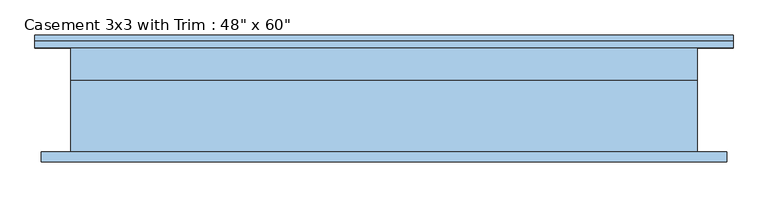
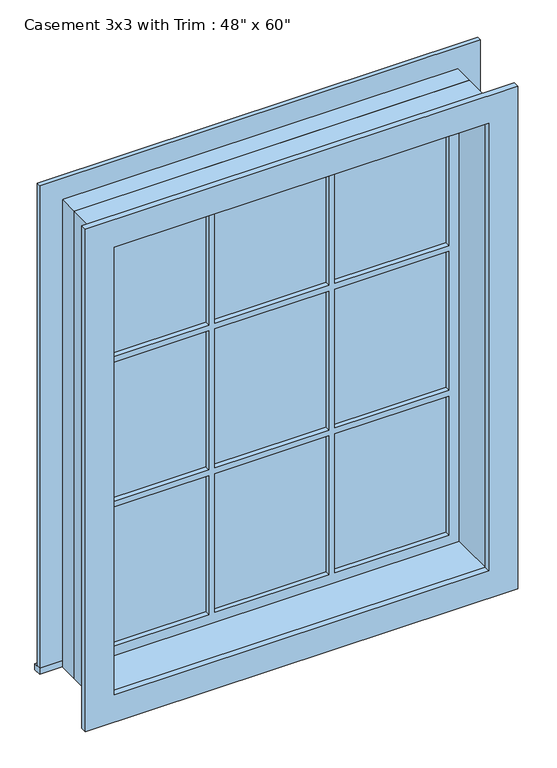
"""IFC4 building model written with IfcOpenShell, lengths in millimetres: window geometry."""

from ifc_helpers import new_model, si_unit, frame, origin, place, context, project, spatial, polyline, outline, extrude, source, transform, mapped, element, save


def window_cfa1ffdd(model_context):
    return source(origin(), model_context, "Body", "SweptSolid", [
        extrude(outline(polyline([(-679.45, 127.0), (679.45, 127.0), (679.45, 101.6), (-679.45, 101.6), (-679.45, 127.0)])), frame((0.0, 0.0, 609.6), z_axis=(0.0, 0.0, 1.0), x_axis=(1.0, 0.0, 0.0)), (0.0, 0.0, 1.0), 19.05),
        extrude(outline(polyline([(2114.55, -590.55), (2114.55, 590.55), (628.65, 590.55), (628.65, 679.45), (2203.45, 679.45), (2203.45, -679.45), (628.65, -679.45), (628.65, -590.55), (2114.55, -590.55)])), frame((0.0, 101.6, 0.0), z_axis=(0.0, 1.0, 0.0), x_axis=(0.0, 0.0, 1.0)), (0.0, 0.0, 1.0), 12.7),
        extrude(outline(polyline([(194.7333333, 66.675), (546.1, 66.675), (546.1, 53.975), (194.7333333, 53.975), (194.7333333, 66.675)])), frame((0.0, 0.0, 1617.1333333), z_axis=(0.0, 0.0, 1.0), x_axis=(1.0, 0.0, 0.0)), (0.0, 0.0, 1.0), 452.9666667),
        extrude(outline(polyline([(-175.6833333, 66.675), (175.6833333, 66.675), (175.6833333, 53.975), (-175.6833333, 53.975), (-175.6833333, 66.675)])), frame((0.0, 0.0, 1617.1333333), z_axis=(0.0, 0.0, 1.0), x_axis=(1.0, 0.0, 0.0)), (0.0, 0.0, 1.0), 452.9666667),
        extrude(outline(polyline([(-546.1, 66.675), (-194.7333333, 66.675), (-194.7333333, 53.975), (-546.1, 53.975), (-546.1, 66.675)])), frame((0.0, 0.0, 1617.1333333), z_axis=(0.0, 0.0, 1.0), x_axis=(1.0, 0.0, 0.0)), (0.0, 0.0, 1.0), 452.9666667),
        extrude(outline(polyline([(-546.1, 66.675), (-194.7333333, 66.675), (-194.7333333, 53.975), (-546.1, 53.975), (-546.1, 66.675)])), frame((0.0, 0.0, 1145.1166667), z_axis=(0.0, 0.0, 1.0), x_axis=(1.0, 0.0, 0.0)), (0.0, 0.0, 1.0), 452.9666667),
        extrude(outline(polyline([(-175.6833333, 66.675), (175.6833333, 66.675), (175.6833333, 53.975), (-175.6833333, 53.975), (-175.6833333, 66.675)])), frame((0.0, 0.0, 1145.1166667), z_axis=(0.0, 0.0, 1.0), x_axis=(1.0, 0.0, 0.0)), (0.0, 0.0, 1.0), 452.9666667),
        extrude(outline(polyline([(194.7333333, 66.675), (546.1, 66.675), (546.1, 53.975), (194.7333333, 53.975), (194.7333333, 66.675)])), frame((0.0, 0.0, 1145.1166667), z_axis=(0.0, 0.0, 1.0), x_axis=(1.0, 0.0, 0.0)), (0.0, 0.0, 1.0), 452.9666667),
        extrude(outline(polyline([(194.7333333, 66.675), (546.1, 66.675), (546.1, 53.975), (194.7333333, 53.975), (194.7333333, 66.675)])), frame((0.0, 0.0, 673.1), z_axis=(0.0, 0.0, 1.0), x_axis=(1.0, 0.0, 0.0)), (0.0, 0.0, 1.0), 452.9666667),
        extrude(outline(polyline([(-175.6833333, 66.675), (175.6833333, 66.675), (175.6833333, 53.975), (-175.6833333, 53.975), (-175.6833333, 66.675)])), frame((0.0, 0.0, 673.1), z_axis=(0.0, 0.0, 1.0), x_axis=(1.0, 0.0, 0.0)), (0.0, 0.0, 1.0), 452.9666667),
        extrude(outline(polyline([(-546.1, 66.675), (-194.7333333, 66.675), (-194.7333333, 53.975), (-546.1, 53.975), (-546.1, 66.675)])), frame((0.0, 0.0, 673.1), z_axis=(0.0, 0.0, 1.0), x_axis=(1.0, 0.0, 0.0)), (0.0, 0.0, 1.0), 452.9666667),
        extrude(outline(polyline([(2190.75, 666.75), (2190.75, -666.75), (552.45, -666.75), (552.45, 666.75), (2190.75, 666.75)]), holes=[polyline([(2101.85, 577.85), (641.35, 577.85), (641.35, -577.85), (2101.85, -577.85), (2101.85, 577.85)])]), frame((0.0, -120.65, 0.0), z_axis=(0.0, 1.0, 0.0), x_axis=(0.0, 0.0, 1.0)), (0.0, 0.0, 1.0), 19.05),
        extrude(outline(polyline([(2114.55, -590.55), (628.65, -590.55), (628.65, 590.55), (2114.55, 590.55), (2114.55, -590.55)]), holes=[polyline([(2070.1, -194.7333333), (1617.1333333, -194.7333333), (1617.1333333, -546.1), (2070.1, -546.1), (2070.1, -194.7333333)]), polyline([(1598.0833333, -194.7333333), (1145.1166667, -194.7333333), (1145.1166667, -546.1), (1598.0833333, -546.1), (1598.0833333, -194.7333333)]), polyline([(1126.0666667, -194.7333333), (673.1, -194.7333333), (673.1, -546.1), (1126.0666667, -546.1), (1126.0666667, -194.7333333)]), polyline([(2070.1, 175.6833333), (1617.1333333, 175.6833333), (1617.1333333, -175.6833333), (2070.1, -175.6833333), (2070.1, 175.6833333)]), polyline([(1598.0833333, 175.6833333), (1145.1166667, 175.6833333), (1145.1166667, -175.6833333), (1598.0833333, -175.6833333), (1598.0833333, 175.6833333)]), polyline([(1126.0666667, 175.6833333), (673.1, 175.6833333), (673.1, -175.6833333), (1126.0666667, -175.6833333), (1126.0666667, 175.6833333)]), polyline([(2070.1, 546.1), (1617.1333333, 546.1), (1617.1333333, 194.7333333), (2070.1, 194.7333333), (2070.1, 546.1)]), polyline([(1598.0833333, 546.1), (1145.1166667, 546.1), (1145.1166667, 194.7333333), (1598.0833333, 194.7333333), (1598.0833333, 546.1)]), polyline([(1126.0666667, 546.1), (673.1, 546.1), (673.1, 194.7333333), (1126.0666667, 194.7333333), (1126.0666667, 546.1)])]), frame((0.0, 38.1, 0.0), z_axis=(0.0, 1.0, 0.0), x_axis=(0.0, 0.0, 1.0)), (0.0, 0.0, 1.0), 44.45),
        extrude(outline(polyline([(2133.6, -609.6), (609.6, -609.6), (609.6, 609.6), (2133.6, 609.6), (2133.6, -609.6)]), holes=[polyline([(2101.85, -577.85), (2101.85, 577.85), (641.35, 577.85), (641.35, -577.85), (2101.85, -577.85)])]), frame((0.0, -101.6, 0.0), z_axis=(0.0, 1.0, 0.0), x_axis=(0.0, 0.0, 1.0)), (0.0, 0.0, 1.0), 139.7),
        extrude(outline(polyline([(2133.6, 609.6), (2133.6, -609.6), (609.6, -609.6), (609.6, 609.6), (2133.6, 609.6)]), holes=[polyline([(2114.55, 590.55), (628.65, 590.55), (628.65, -590.55), (2114.55, -590.55), (2114.55, 590.55)])]), frame((0.0, 38.1, 0.0), z_axis=(0.0, 1.0, 0.0), x_axis=(0.0, 0.0, 1.0)), (0.0, 0.0, 1.0), 63.5),
    ])


if __name__ == "__main__":
    model = new_model("IFC4")
    model_context = context("Model", 3, world=origin())
    ifc_project = project(units=[si_unit("LENGTHUNIT", "METRE", prefix="MILLI")], contexts=[model_context])
    site = spatial("IfcSite", under=ifc_project)
    building = spatial("IfcBuilding", under=site)
    placement = place(None, origin())
    window_shape = window_cfa1ffdd(model_context)
    element("IfcWindow", 1, ObjectType="Casement 3x3 with Trim : 48\" x 60\"", at=placement, inside=building, context=model_context, shape_type="MappedRepresentation", body=[
        mapped(window_shape, transform((0.0, 0.0, 0.0), x_axis=(1.0, 0.0, 0.0), y_axis=(0.0, 1.0, 0.0), z_axis=(0.0, 0.0, 1.0))),
    ])
    save(model, "model.ifc")

# Revit data of these elements
# Type "Casement 3x3 with Trim : 48\" x 60\""
#   Type Mark = "11"
#   Construction Type Id = "GSP4R"
#   Assembly Code = "B2020100"
#   Analytic Construction = "1/8 in Pilkington single glazing"
#   Visual Light Transmittance = 0.9
#   Solar Heat Gain Coefficient = 0.78
#   Heat Transfer Coefficient (U) = 0.6496 BTU/(h·ft²·°F)
#   Height = 5' - 0"
#   Default Sill Height = 2' - 0"
#   Trim Projection - Ext. = 0' - 0 1/2"
#   Trim Projection - Int. = 0' - 0 3/4"
#   Trim Width - Exterior = 0' - 3 1/2"
#   Trim Width - Interior = 0' - 3 1/2"
#   Width = 4' - 0"
#   Window Inset = 0' - 0 3/4"
#   Define Thermal Properties by = 1
#   Glass Pane Material = Glass
#   Sash Material = Sash
#   Trim Exterior Material = Trim
#   Trim Interior Material = Trim
#   Wall Closure = (empty or 0)
# Element 1 (IfcWindow, "Casement 3x3 with Trim : 48\" x 60\"")
#   Materials on its faces: "Sash", "Glass", "Trim"
# Materials
#   "Glass": class "Glass", colour RGB 0 128 192, transparency 0.75, Description = "Soda Lime Glass", Cost = 0
#   "Sash": class "Wood", colour RGB 224 178 126, transparency 0
#   "Trim": class "Wood", colour RGB 224 178 126, transparency 0
